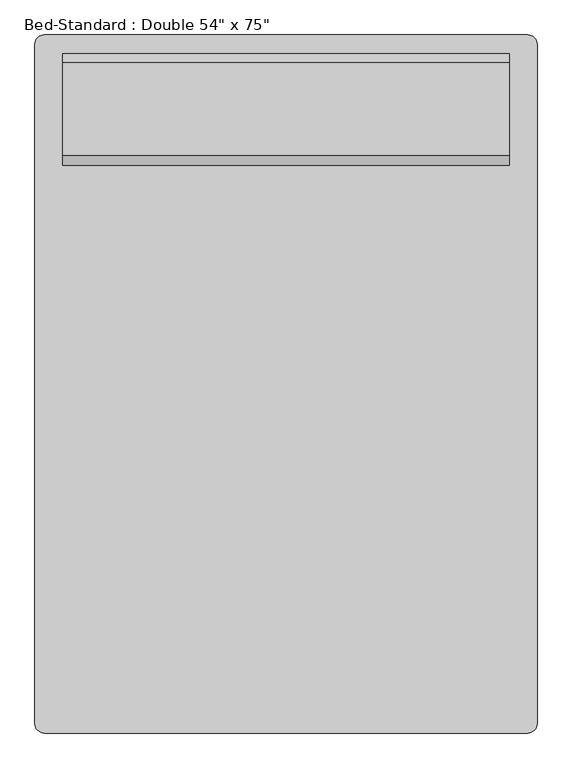
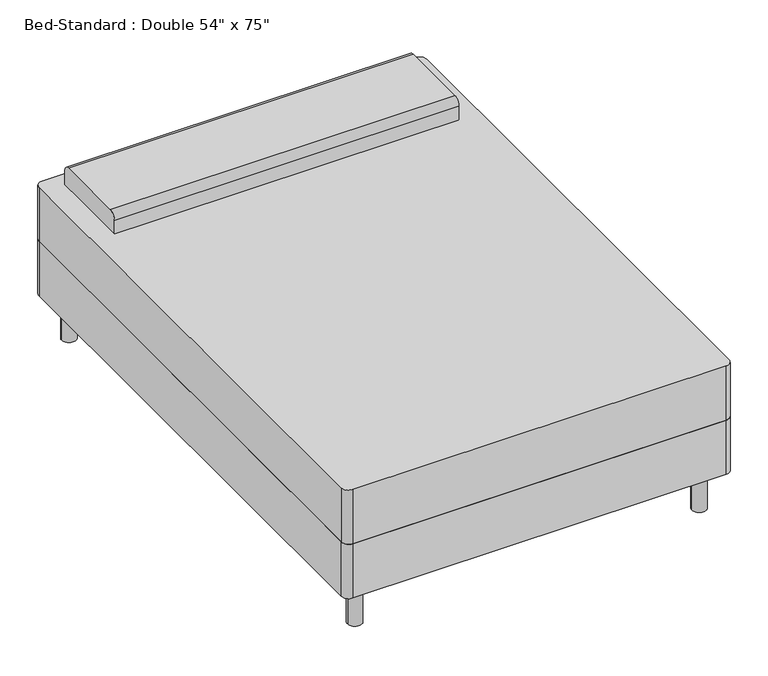
"""IFC4 building model written with IfcOpenShell, lengths in millimetres: furniture geometry."""

from ifc_helpers import new_model, si_unit, point, frame, frame_2d, origin, origin_with_axes, place, context, project, spatial, polyline, circle_curve, trimmed, segment, composite_curve, outline, extrude, source, transform, mapped, element, save


def furniture_0253826f(model_context):
    return source(origin(), model_context, "Body", "SweptSolid", [
        extrude(outline(composite_curve([segment(polyline([(-414.3114754, -972.695082), (-414.3114754, 881.504918)]), True, "CONTINUOUS"), segment(trimmed(circle_curve(frame_2d((-388.9114754, 881.504918)), 25.4), [point((-414.3114754, 881.504918))], [point((-388.9114754, 906.904918))], False, "CARTESIAN"), True, "CONTINUOUS"), segment(polyline([(-388.9114754, 906.904918), (931.8885246, 906.904918)]), True, "CONTINUOUS"), segment(trimmed(circle_curve(frame_2d((931.8885246, 881.504918)), 25.4), [point((931.8885246, 906.904918))], [point((957.2885246, 881.504918))], False, "CARTESIAN"), True, "CONTINUOUS"), segment(polyline([(957.2885246, 881.504918), (957.2885246, -972.695082)]), True, "CONTINUOUS"), segment(trimmed(circle_curve(frame_2d((931.8885246, -972.695082)), 25.4), [point((957.2885246, -972.695082))], [point((931.8885246, -998.095082))], False, "CARTESIAN"), True, "CONTINUOUS"), segment(polyline([(931.8885246, -998.095082), (-388.9114754, -998.095082)]), True, "CONTINUOUS"), segment(trimmed(circle_curve(frame_2d((-388.9114754, -972.695082)), 25.4), [point((-388.9114754, -998.095082))], [point((-414.3114754, -972.695082))], False, "CARTESIAN"), True, "CONTINUOUS")], self_intersect=False)), frame((0.0, 0.0, 152.4), z_axis=(0.0, 0.0, 1.0), x_axis=(1.0, 0.0, 0.0)), (0.0, 0.0, 1.0), 203.2),
        extrude(outline(composite_curve([segment(polyline([(551.304918, 558.8), (551.304918, 609.6)]), True, "CONTINUOUS"), segment(trimmed(circle_curve(frame_2d((576.704918, 609.6)), 25.4), [point((551.304918, 609.6))], [point((576.704918, 635.0))], False, "CARTESIAN"), True, "CONTINUOUS"), segment(polyline([(576.704918, 635.0), (830.704918, 635.0)]), True, "CONTINUOUS"), segment(trimmed(circle_curve(frame_2d((830.704918, 609.6)), 25.4), [point((830.704918, 635.0))], [point((856.104918, 609.6))], False, "CARTESIAN"), True, "CONTINUOUS"), segment(polyline([(856.104918, 609.6), (856.104918, 558.8), (551.304918, 558.8)]), True, "CONTINUOUS")], self_intersect=False)), frame((-338.1114754, 0.0, 0.0), z_axis=(1.0, 0.0, 0.0), x_axis=(0.0, 1.0, 0.0)), (0.0, 0.0, 1.0), 1219.2),
        extrude(outline(composite_curve([segment(trimmed(circle_curve(frame_2d((-338.1114754, 830.704918)), 25.4), [point((-363.5114754, 830.704918))], [point((-312.7114754, 830.704918))], False, "CARTESIAN"), True, "CONTINUOUS"), segment(trimmed(circle_curve(frame_2d((-338.1114754, 830.704918)), 25.4), [point((-312.7114754, 830.704918))], [point((-363.5114754, 830.704918))], False, "CARTESIAN"), True, "CONTINUOUS")], self_intersect=False)), origin_with_axes(), (0.0, 0.0, 1.0), 152.4),
        extrude(outline(composite_curve([segment(trimmed(circle_curve(frame_2d((881.0885246, 830.704918)), 25.4), [point((855.6885246, 830.704918))], [point((906.4885246, 830.704918))], False, "CARTESIAN"), True, "CONTINUOUS"), segment(trimmed(circle_curve(frame_2d((881.0885246, 830.704918)), 25.4), [point((906.4885246, 830.704918))], [point((855.6885246, 830.704918))], False, "CARTESIAN"), True, "CONTINUOUS")], self_intersect=False)), origin_with_axes(), (0.0, 0.0, 1.0), 152.4),
        extrude(outline(composite_curve([segment(trimmed(circle_curve(frame_2d((881.0885246, -921.895082)), 25.4), [point((855.6885246, -921.895082))], [point((906.4885246, -921.895082))], False, "CARTESIAN"), True, "CONTINUOUS"), segment(trimmed(circle_curve(frame_2d((881.0885246, -921.895082)), 25.4), [point((906.4885246, -921.895082))], [point((855.6885246, -921.895082))], False, "CARTESIAN"), True, "CONTINUOUS")], self_intersect=False)), origin_with_axes(), (0.0, 0.0, 1.0), 152.4),
        extrude(outline(composite_curve([segment(trimmed(circle_curve(frame_2d((-338.1114754, -921.895082)), 25.4), [point((-363.5114754, -921.895082))], [point((-312.7114754, -921.895082))], False, "CARTESIAN"), True, "CONTINUOUS"), segment(trimmed(circle_curve(frame_2d((-338.1114754, -921.895082)), 25.4), [point((-312.7114754, -921.895082))], [point((-363.5114754, -921.895082))], False, "CARTESIAN"), True, "CONTINUOUS")], self_intersect=False)), origin_with_axes(), (0.0, 0.0, 1.0), 152.4),
        extrude(outline(composite_curve([segment(polyline([(-388.9114754, 906.904918), (931.8885246, 906.904918)]), True, "CONTINUOUS"), segment(trimmed(circle_curve(frame_2d((931.8885246, 881.504918)), 25.4), [point((931.8885246, 906.904918))], [point((957.2885246, 881.504918))], False, "CARTESIAN"), True, "CONTINUOUS"), segment(polyline([(957.2885246, 881.504918), (957.2885246, -972.695082)]), True, "CONTINUOUS"), segment(trimmed(circle_curve(frame_2d((931.8885246, -972.695082)), 25.4), [point((957.2885246, -972.695082))], [point((931.8885246, -998.095082))], False, "CARTESIAN"), True, "CONTINUOUS"), segment(polyline([(931.8885246, -998.095082), (-388.9114754, -998.095082)]), True, "CONTINUOUS"), segment(trimmed(circle_curve(frame_2d((-388.9114754, -972.695082)), 25.4), [point((-388.9114754, -998.095082))], [point((-414.3114754, -972.695082))], False, "CARTESIAN"), True, "CONTINUOUS"), segment(polyline([(-414.3114754, -972.695082), (-414.3114754, 881.504918)]), True, "CONTINUOUS"), segment(trimmed(circle_curve(frame_2d((-388.9114754, 881.504918)), 25.4), [point((-414.3114754, 881.504918))], [point((-388.9114754, 906.904918))], False, "CARTESIAN"), True, "CONTINUOUS")], self_intersect=False)), frame((0.0, 0.0, 355.6), z_axis=(0.0, 0.0, 1.0), x_axis=(1.0, 0.0, 0.0)), (0.0, 0.0, 1.0), 203.2),
    ])


if __name__ == "__main__":
    model = new_model("IFC4")
    model_context = context("Model", 3, world=origin())
    ifc_project = project(units=[si_unit("LENGTHUNIT", "METRE", prefix="MILLI")], contexts=[model_context])
    site = spatial("IfcSite", under=ifc_project)
    building = spatial("IfcBuilding", under=site)
    placement = place(None, origin())
    furniture_shape = furniture_0253826f(model_context)
    element("IfcFurniture", 1, ObjectType="Bed-Standard : Double 54\" x 75\"", at=placement, inside=building, context=model_context, shape_type="MappedRepresentation", body=[
        mapped(furniture_shape, transform((0.0, 0.0, 0.0), x_axis=(1.0, 0.0, 0.0), y_axis=(0.0, 1.0, 0.0), z_axis=(0.0, 0.0, 1.0))),
    ])
    save(model, "model.ifc")

# Revit data of these elements
# Type "Bed-Standard : Double 54\" x 75\""
#   Assembly Code = "E2020200"
#   Length = 6' - 3"
#   Width = 4' - 6"
#   Leg Material = Steel, Chrome Plated
#   Mattress Material = Oak Flooring
#   Default Elevation = 0
# Element 1 (IfcFurniture, "Bed-Standard : Double 54\" x 75\"")
#   Materials on its faces: "Linen, White", "Steel, Chrome Plated"
# Materials
#   "Steel, Chrome Plated": class "Metal", colour RGB 17 17 17, transparency 0, Description = "Chromiuim plated steel", Cost = 0
#   "Oak Flooring": class "Wood", colour RGB 216 169 114, transparency 0, Description = "Quercus Rubra", Cost = 0
#   "Linen, White": class "Textile", colour RGB 247 247 239, transparency 0, Description = "Linen, white", Cost = 0
